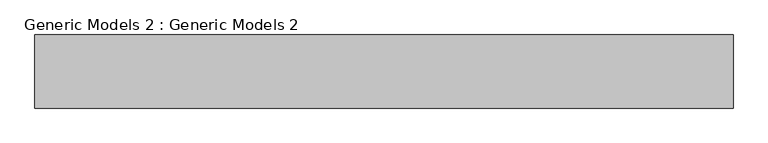
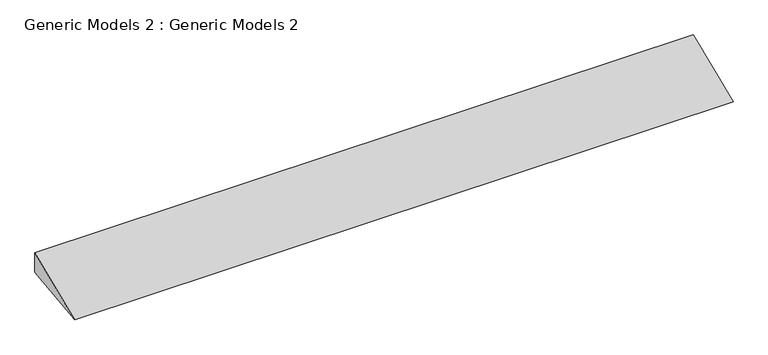
"""IFC4 building model written with IfcOpenShell, lengths in millimetres: proxy geometry, Generic Models 2 : Generic Models 2."""

from ifc_helpers import new_model, si_unit, frame, origin, place, context, project, spatial, polyline, outline, extrude, source, transform, mapped, element, save


def generic_models_2_generic_models_2_23ebf3b1(model_context):
    return source(origin(), model_context, "Body", "SweptSolid", [
        extrude(outline(polyline([(-4568.8893014, -217.5067423), (-4052.3758122, 0.0), (-4052.3758122, -152.4), (-4568.8893014, -217.5067423)])), frame((5486.7916032, 0.0, 0.0), z_axis=(1.0, 0.0, 0.0), x_axis=(0.0, 1.0, 0.0)), (0.0, 0.0, 1.0), 4933.2822872),
    ])


if __name__ == "__main__":
    model = new_model("IFC4")
    model_context = context("Model", 3, world=origin())
    ifc_project = project(units=[si_unit("LENGTHUNIT", "METRE", prefix="MILLI")], contexts=[model_context])
    site = spatial("IfcSite", under=ifc_project)
    building = spatial("IfcBuilding", under=site)
    placement = place(None, origin())
    generic_models_2_generic_models_2_shape = generic_models_2_generic_models_2_23ebf3b1(model_context)
    element("IfcBuildingElementProxy", 1, Name="Generic Models 2 : Generic Models 2", ObjectType="Generic Models 2 : Generic Models 2", at=placement, inside=building, context=model_context, shape_type="MappedRepresentation", body=[
        mapped(generic_models_2_generic_models_2_shape, transform((0.0, 0.0, 0.0), x_axis=(1.0, 0.0, 0.0), y_axis=(0.0, 1.0, 0.0), z_axis=(0.0, 0.0, 1.0))),
    ])
    save(model, "model.ifc")
